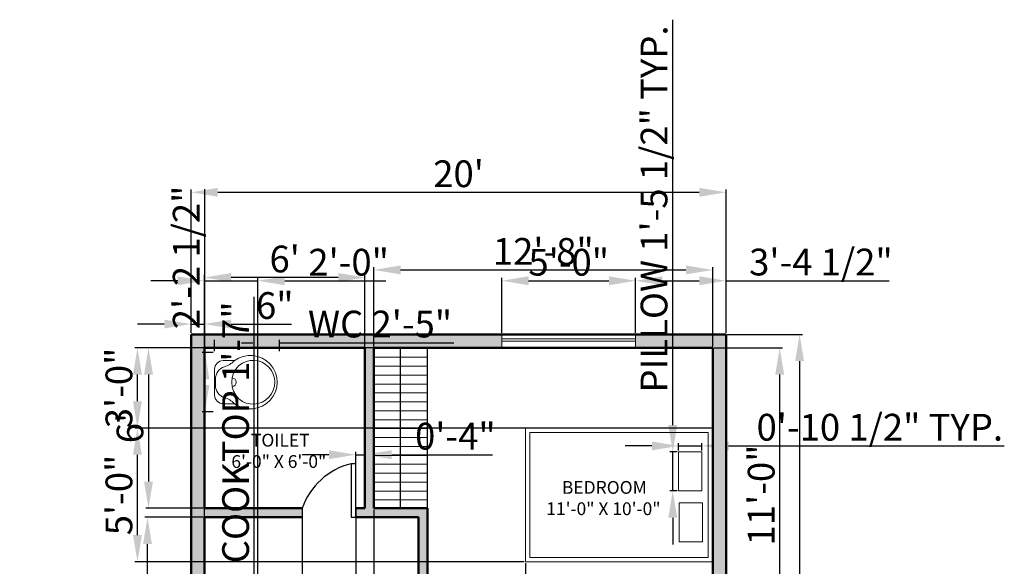
# Model space of a CAD drawing. Units: inches. Extents: x 2549 to 2991, y 1646 to 2183.
# Tile 3 of 3: x 2549 to 2991, y 1938 to 2183. Entities that reach past the tile are written whole.
import ezdxf

# ---------------------------------------------------------------- set-up
doc = ezdxf.new("R2010")
doc.units = ezdxf.units.IN
for name, color, linetype, lineweight in [('A-ANNO-DIMS', 2, 'Continuous', 18), ('A-AREA-IDEN', 7, 'Continuous', 25), ('A-DOOR', 3, 'Continuous', 25), ('A-FLOR-CASE', 8, 'Continuous', 25), ('A-FLOR-FIXT', 8, 'Continuous', 20), ('A-FLOR-PATT', 9, 'Continuous', 13), ('A-FURN', 9, 'Continuous', 18), ('A-GLAZ', 4, 'Continuous', 18), ('A-WALL', 7, 'Continuous', 50)]:
    doc.layers.add(name, color=color, linetype=linetype, lineweight=lineweight)
doc.layers.add('A-WALL-PATT', color=251, linetype='Continuous', lineweight=13, true_color=0x636466)
doc.styles.get("Standard").update_dxf_attribs({"font": 'arial.ttf'})
doc.dimstyles.new('ISO-25', dxfattribs={"dimtxt": 12, "dimasz": 12, "dimexe": 1.25, "dimexo": 0.625, "dimtad": 1, "dimlunit": 3, "dimtxsty": 'Standard', "dimcen": 2.5, "dimadec": 0, "dimazin": 0, "dimtfac": 1, "dimtmove": 0, "dimatfit": 3, "dimfxl": 1, "dimarcsym": 0})

# ---------------------------------------------------------------- blocks, each defined once
blk = doc.blocks.new('A$C6EF51710')
at = {"linetype": 'ByBlock'}
for p, q in [((0, 0.0811), (0, 0.2335)), ((0.0508, 0.2843), (0.1169, 0.2843)), ((0.0041, 0.1392), (0.0041, 0.1755)), ((0.1169, 0.0303), (0.0508, 0.0303))]:
    blk.add_line(p, q, dxfattribs=at)
for centre, radius, start, end in [((0.2107, 0.1573), 0.1576, 232.89836, 127.10164), ((0.0508, 0.2335), 0.0508, 90, 180), ((0.0803, 0.1755), 0.0762, 107.10464, 180), ((0.0168, 0.3818), 0.1397, 287.10464, 315), ((0.2413, 0.1573), 0.1397, 135, 225), ((0.2254, 0.1573), 0.1289, 230.00836, 129.99164), ((0.1016, 0.1573), 0.0254, 275.21591, 84.78409), ((0.0803, 0.1392), 0.0762, 180, 252.89536), ((0.0508, 0.0811), 0.0508, 180, 270), ((0.0168, -0.0672), 0.1397, 45, 72.89536)]:
    blk.add_arc(centre, radius, start, end, dxfattribs=at)
blk = doc.blocks.new('*D5')
at = {"layer": 'A-ANNO-DIMS', "color": 0, "lineweight": -2, "transparency": 16777216}
for p, q in [((2866.66, 2042.26), (2900.26, 2042.26)), ((2899.01, 2030.26), (2899.01, 1694.26)), ((2866.66, 1682.26), (2900.26, 1682.26))]:
    blk.add_line(p, q, dxfattribs=at)
at = {"layer": 'A-ANNO-DIMS', "color": 0, "transparency": 16777216}
for points in [[(2897.01, 2030.26), (2901.01, 2030.26), (2899.01, 2042.26)], [(2897.01, 1694.26), (2901.01, 1694.26), (2899.01, 1682.26)]]:
    blk.add_solid(points, dxfattribs=at)
at = {"layer": 'Defpoints', "color": 0, "transparency": 16777216}
for p in [(2866.04, 2042.26), (2866.04, 1682.26), (2899.01, 1682.26)]:
    blk.add_point(p, dxfattribs=at)
at = {"layer": 'A-ANNO-DIMS', "color": 0, "transparency": 16777216, "insert": (2892.25, 1862.26), "char_height": 12, "attachment_point": 5, "rotation": 90}
blk.add_mtext("30'", dxfattribs=at)
blk = doc.blocks.new('*D6')
at = {"layer": 'A-ANNO-DIMS', "color": 0, "lineweight": -2, "transparency": 16777216}
for p, q in [((2626.04, 2042.89), (2626.04, 2107.23)), ((2866.04, 2042.89), (2866.04, 2107.23)), ((2638.04, 2105.98), (2854.04, 2105.98))]:
    blk.add_line(p, q, dxfattribs=at)
at = {"layer": 'A-ANNO-DIMS', "color": 0, "transparency": 16777216}
for points in [[(2638.04, 2107.98), (2638.04, 2103.98), (2626.04, 2105.98)], [(2854.04, 2107.98), (2854.04, 2103.98), (2866.04, 2105.98)]]:
    blk.add_solid(points, dxfattribs=at)
at = {"layer": 'Defpoints', "color": 0, "transparency": 16777216}
for p in [(2866.04, 2105.98), (2626.04, 2042.26), (2866.04, 2042.26)]:
    blk.add_point(p, dxfattribs=at)
at = {"layer": 'A-ANNO-DIMS', "color": 0, "transparency": 16777216, "insert": (2746.04, 2112.74), "char_height": 12, "attachment_point": 5}
blk.add_mtext("20'", dxfattribs=at)
blk = doc.blocks.new('*D7')
at = {"layer": 'A-ANNO-DIMS', "color": 0, "lineweight": -2, "transparency": 16777216}
for p, q in [((2708.04, 2036.89), (2708.04, 2072.42)), ((2860.04, 2036.89), (2860.04, 2072.42)), ((2720.04, 2071.17), (2848.04, 2071.17))]:
    blk.add_line(p, q, dxfattribs=at)
at = {"layer": 'A-ANNO-DIMS', "color": 0, "transparency": 16777216}
for points in [[(2720.04, 2073.17), (2720.04, 2069.17), (2708.04, 2071.17)], [(2848.04, 2073.17), (2848.04, 2069.17), (2860.04, 2071.17)]]:
    blk.add_solid(points, dxfattribs=at)
at = {"layer": 'Defpoints', "color": 0, "transparency": 16777216}
for p in [(2860.04, 2071.17), (2708.04, 2036.26), (2860.04, 2036.26)]:
    blk.add_point(p, dxfattribs=at)
at = {"layer": 'A-ANNO-DIMS', "color": 0, "transparency": 16777216, "insert": (2784.04, 2077.93), "char_height": 12, "attachment_point": 5}
blk.add_mtext('12\'-8"', dxfattribs=at)
blk = doc.blocks.new('*D8')
at = {"layer": 'A-ANNO-DIMS', "color": 0, "lineweight": -2, "transparency": 16777216}
for p, q in [((2632.04, 2036.89), (2632.04, 2069.02)), ((2692.04, 2067.77), (2644.04, 2067.77)), ((2704.04, 2036.89), (2704.04, 2069.02))]:
    blk.add_line(p, q, dxfattribs=at)
at = {"layer": 'A-ANNO-DIMS', "color": 0, "transparency": 16777216}
for points in [[(2644.04, 2069.77), (2644.04, 2065.77), (2632.04, 2067.77)], [(2692.04, 2069.77), (2692.04, 2065.77), (2704.04, 2067.77)]]:
    blk.add_solid(points, dxfattribs=at)
at = {"layer": 'Defpoints', "color": 0, "transparency": 16777216}
for p in [(2632.04, 2067.77), (2632.04, 2036.26), (2704.04, 2036.26)]:
    blk.add_point(p, dxfattribs=at)
at = {"layer": 'A-ANNO-DIMS', "color": 0, "transparency": 16777216, "insert": (2668.04, 2074.52), "char_height": 12, "attachment_point": 5}
blk.add_mtext("6'", dxfattribs=at)
blk = doc.blocks.new('*D9')
at = {"layer": 'A-ANNO-DIMS', "color": 0, "lineweight": -2, "transparency": 16777216}
for p, q in [((2614.04, 2046.9), (2602.04, 2046.9)), ((2626.04, 2042.89), (2626.04, 2048.15)), ((2626.04, 2046.9), (2632.04, 2046.9)), ((2632.04, 2042.89), (2632.04, 2048.15)), ((2644.04, 2046.9), (2671.15, 2046.9))]:
    blk.add_line(p, q, dxfattribs=at)
at = {"layer": 'A-ANNO-DIMS', "color": 0, "transparency": 16777216}
for points in [[(2614.04, 2048.9), (2614.04, 2044.9), (2626.04, 2046.9)], [(2644.04, 2048.9), (2644.04, 2044.9), (2632.04, 2046.9)]]:
    blk.add_solid(points, dxfattribs=at)
at = {"layer": 'Defpoints', "color": 0, "transparency": 16777216}
for p in [(2632.04, 2046.9), (2626.04, 2042.26), (2632.04, 2042.26)]:
    blk.add_point(p, dxfattribs=at)
at = {"layer": 'A-ANNO-DIMS', "color": 0, "transparency": 16777216, "insert": (2663.59, 2053.65), "char_height": 12, "attachment_point": 5}
blk.add_mtext('6"', dxfattribs=at)
blk = doc.blocks.new('*D10')
at = {"layer": 'A-ANNO-DIMS', "color": 0, "lineweight": -2, "transparency": 16777216}
for p, q in [((2631.41, 2036.26), (2605.7, 2036.26)), ((2606.95, 2024.26), (2606.95, 1976.26)), ((2631.41, 1964.26), (2605.7, 1964.26))]:
    blk.add_line(p, q, dxfattribs=at)
at = {"layer": 'A-ANNO-DIMS', "color": 0, "transparency": 16777216}
for points in [[(2604.95, 2024.26), (2608.95, 2024.26), (2606.95, 2036.26)], [(2604.95, 1976.26), (2608.95, 1976.26), (2606.95, 1964.26)]]:
    blk.add_solid(points, dxfattribs=at)
at = {"layer": 'Defpoints', "color": 0, "transparency": 16777216}
for p in [(2632.04, 2036.26), (2606.95, 1964.26), (2632.04, 1964.26)]:
    blk.add_point(p, dxfattribs=at)
at = {"layer": 'A-ANNO-DIMS', "color": 0, "transparency": 16777216, "insert": (2600.19, 2000.26), "char_height": 12, "attachment_point": 5, "rotation": 90}
blk.add_mtext("6'", dxfattribs=at)
blk = doc.blocks.new('*D11')
at = {"layer": 'A-ANNO-DIMS', "color": 0, "lineweight": -2, "transparency": 16777216}
for p, q in [((2631.41, 1960.26), (2605.25, 1960.26)), ((2606.5, 1832.26), (2606.5, 1948.26)), ((2631.41, 1820.26), (2605.25, 1820.26))]:
    blk.add_line(p, q, dxfattribs=at)
at = {"layer": 'A-ANNO-DIMS', "color": 0, "transparency": 16777216}
for points in [[(2604.5, 1948.26), (2608.5, 1948.26), (2606.5, 1960.26)], [(2604.5, 1832.26), (2608.5, 1832.26), (2606.5, 1820.26)]]:
    blk.add_solid(points, dxfattribs=at)
at = {"layer": 'Defpoints', "color": 0, "transparency": 16777216}
for p in [(2606.5, 1960.26), (2632.04, 1960.26), (2632.04, 1820.26)]:
    blk.add_point(p, dxfattribs=at)
at = {"layer": 'A-ANNO-DIMS', "color": 0, "transparency": 16777216, "insert": (2599.75, 1890.26), "char_height": 12, "attachment_point": 5, "rotation": 90}
blk.add_mtext('11\'-8"', dxfattribs=at)
blk = doc.blocks.new('BED-PILLOW')
blk.add_lwpolyline([(0, 17.55), (10.43, 17.55), (10.43, 0), (0, 0)], close=True)
blk = doc.blocks.new('*D20')
at = {"layer": 'A-ANNO-DIMS', "color": 0, "lineweight": -2, "transparency": 16777216}
for p, q in [((2842.11, 2001.62), (2842.11, 2183.39)), ((2844.12, 1989.62), (2840.86, 1989.62)), ((2842.11, 1972.07), (2842.11, 1989.62)), ((2844.12, 1972.07), (2840.86, 1972.07)), ((2842.11, 1960.07), (2842.11, 1948.07))]:
    blk.add_line(p, q, dxfattribs=at)
at = {"layer": 'A-ANNO-DIMS', "color": 0, "transparency": 16777216}
for points in [[(2840.11, 2001.62), (2844.11, 2001.62), (2842.11, 1989.62)], [(2840.11, 1960.07), (2844.11, 1960.07), (2842.11, 1972.07)]]:
    blk.add_solid(points, dxfattribs=at)
at = {"layer": 'Defpoints', "color": 0, "transparency": 16777216}
for p in [(2842.11, 1989.62), (2844.74, 1989.62), (2844.74, 1972.07)]:
    blk.add_point(p, dxfattribs=at)
at = {"layer": 'A-ANNO-DIMS', "color": 0, "transparency": 16777216, "insert": (2835.28, 2098.5), "char_height": 12, "attachment_point": 5, "rotation": 90}
blk.add_mtext('PILLOW 1\'-5 1/2" TYP.', dxfattribs=at)
blk = doc.blocks.new('*D21')
at = {"layer": 'A-ANNO-DIMS', "color": 0, "lineweight": -2, "transparency": 16777216}
for p, q in [((2832.74, 1992.25), (2820.74, 1992.25)), ((2844.74, 1990.25), (2844.74, 1993.5)), ((2844.74, 1992.25), (2855.17, 1992.25)), ((2855.17, 1990.25), (2855.17, 1993.5)), ((2867.17, 1992.25), (2990.85, 1992.25))]:
    blk.add_line(p, q, dxfattribs=at)
at = {"layer": 'A-ANNO-DIMS', "color": 0, "transparency": 16777216}
for points in [[(2832.74, 1994.25), (2832.74, 1990.25), (2844.74, 1992.25)], [(2867.17, 1994.25), (2867.17, 1990.25), (2855.17, 1992.25)]]:
    blk.add_solid(points, dxfattribs=at)
at = {"layer": 'Defpoints', "color": 0, "transparency": 16777216}
for p in [(2855.17, 1992.25), (2844.74, 1989.62), (2855.17, 1989.62)]:
    blk.add_point(p, dxfattribs=at)
at = {"layer": 'A-ANNO-DIMS', "color": 0, "transparency": 16777216, "insert": (2935.01, 1999.08), "char_height": 12, "attachment_point": 5}
blk.add_mtext('0\'-10 1/2" TYP.', dxfattribs=at)
blk = doc.blocks.new('*D24')
at = {"layer": 'A-ANNO-DIMS', "color": 0, "lineweight": -2, "transparency": 16777216}
for p, q in [((2654.4, 1925.59), (2654.4, 2059.08)), ((2652.15, 1913.59), (2655.65, 1913.59)), ((2654.4, 1894.39), (2654.4, 1913.59)), ((2652.15, 1894.39), (2655.65, 1894.39)), ((2654.4, 1882.39), (2654.4, 1870.39))]:
    blk.add_line(p, q, dxfattribs=at)
at = {"layer": 'A-ANNO-DIMS', "color": 0, "transparency": 16777216}
for points in [[(2652.4, 1925.59), (2656.4, 1925.59), (2654.4, 1913.59)], [(2652.4, 1882.39), (2656.4, 1882.39), (2654.4, 1894.39)]]:
    blk.add_solid(points, dxfattribs=at)
at = {"layer": 'Defpoints', "color": 0, "transparency": 16777216}
for p in [(2651.52, 1913.59), (2654.4, 1913.59), (2651.52, 1894.39)]:
    blk.add_point(p, dxfattribs=at)
at = {"layer": 'A-ANNO-DIMS', "color": 0, "transparency": 16777216, "insert": (2647.57, 1998.33), "char_height": 12, "attachment_point": 5, "rotation": 90}
blk.add_mtext('COOKTOP 1\'-7"', dxfattribs=at)
blk = doc.blocks.new('*D25')
at = {"layer": 'A-ANNO-DIMS', "color": 0, "lineweight": -2, "transparency": 16777216}
for p, q in [((2633.92, 1914.21), (2633.92, 1917.72)), ((2651.52, 1914.21), (2651.52, 1917.72)), ((2621.92, 1916.47), (2549.94, 1916.47)), ((2651.52, 1916.47), (2633.92, 1916.47)), ((2663.52, 1916.47), (2675.52, 1916.47))]:
    blk.add_line(p, q, dxfattribs=at)
at = {"layer": 'A-ANNO-DIMS', "color": 0, "transparency": 16777216}
for points in [[(2621.92, 1918.47), (2621.92, 1914.47), (2633.92, 1916.47)], [(2663.52, 1918.47), (2663.52, 1914.47), (2651.52, 1916.47)]]:
    blk.add_solid(points, dxfattribs=at)
at = {"layer": 'Defpoints', "color": 0, "transparency": 16777216}
for p in [(2633.92, 1916.47), (2633.92, 1913.59), (2651.52, 1913.59)]:
    blk.add_point(p, dxfattribs=at)
at = {"layer": 'A-ANNO-DIMS', "color": 0, "transparency": 16777216, "insert": (2579.93, 1923.3), "char_height": 12, "attachment_point": 5}
blk.add_mtext('1\'-5 1/2"', dxfattribs=at)
blk = doc.blocks.new('*D26')
at = {"layer": 'A-ANNO-DIMS', "color": 0, "lineweight": -2, "transparency": 16777216}
for p, q in [((2636.61, 2034.77), (2636.61, 2039.76)), ((2648.61, 2038.51), (2653.7, 2038.51)), ((2665.7, 2034.77), (2665.7, 2039.76)), ((2665.7, 2038.51), (2743.93, 2038.51))]:
    blk.add_line(p, q, dxfattribs=at)
at = {"layer": 'A-ANNO-DIMS', "color": 0, "transparency": 16777216}
for points in [[(2648.61, 2040.51), (2648.61, 2036.51), (2636.61, 2038.51)], [(2653.7, 2040.51), (2653.7, 2036.51), (2665.7, 2038.51)]]:
    blk.add_solid(points, dxfattribs=at)
at = {"layer": 'Defpoints', "color": 0, "transparency": 16777216}
for p in [(2665.7, 2038.51), (2636.61, 2034.14), (2665.7, 2034.14)]:
    blk.add_point(p, dxfattribs=at)
at = {"layer": 'A-ANNO-DIMS', "color": 0, "transparency": 16777216, "insert": (2710.82, 2045.34), "char_height": 12, "attachment_point": 5}
blk.add_mtext('WC 2\'-5"', dxfattribs=at)
blk = doc.blocks.new('*D27')
at = {"layer": 'A-ANNO-DIMS', "color": 0, "lineweight": -2, "transparency": 16777216}
for p, q in [((2632.25, 2034.14), (2632.25, 2107.46)), ((2635.99, 2034.14), (2631, 2034.14)), ((2632.25, 2019.52), (2632.25, 2022.14)), ((2635.99, 2007.52), (2631, 2007.52))]:
    blk.add_line(p, q, dxfattribs=at)
at = {"layer": 'A-ANNO-DIMS', "color": 0, "transparency": 16777216}
for points in [[(2630.25, 2022.14), (2634.25, 2022.14), (2632.25, 2034.14)], [(2630.25, 2019.52), (2634.25, 2019.52), (2632.25, 2007.52)]]:
    blk.add_solid(points, dxfattribs=at)
at = {"layer": 'Defpoints', "color": 0, "transparency": 16777216}
for p in [(2632.25, 2034.14), (2636.61, 2034.14), (2636.61, 2007.52)]:
    blk.add_point(p, dxfattribs=at)
at = {"layer": 'A-ANNO-DIMS', "color": 0, "transparency": 16777216, "insert": (2625.42, 2076.8), "char_height": 12, "attachment_point": 5, "rotation": 90}
blk.add_mtext('2\'-2 1/2"', dxfattribs=at)
blk = doc.blocks.new('*D31')
at = {"layer": 'A-ANNO-DIMS', "color": 0, "lineweight": -2, "transparency": 16777216}
for p, q in [((2765.46, 2042.89), (2765.46, 2067.56)), ((2825.46, 2042.89), (2825.46, 2067.56)), ((2777.46, 2066.31), (2813.46, 2066.31))]:
    blk.add_line(p, q, dxfattribs=at)
at = {"layer": 'A-ANNO-DIMS', "color": 0, "transparency": 16777216}
for points in [[(2777.46, 2068.31), (2777.46, 2064.31), (2765.46, 2066.31)], [(2813.46, 2068.31), (2813.46, 2064.31), (2825.46, 2066.31)]]:
    blk.add_solid(points, dxfattribs=at)
at = {"layer": 'Defpoints', "color": 0, "transparency": 16777216}
for p in [(2825.46, 2066.31), (2765.46, 2042.26), (2825.46, 2042.26)]:
    blk.add_point(p, dxfattribs=at)
at = {"layer": 'A-ANNO-DIMS', "color": 0, "transparency": 16777216, "insert": (2795.46, 2073.07), "char_height": 12, "attachment_point": 5}
blk.add_mtext('5\'-0"', dxfattribs=at)
blk = doc.blocks.new('*D32')
at = {"layer": 'A-ANNO-DIMS', "color": 0, "lineweight": -2, "transparency": 16777216}
for p, q in [((2825.46, 2042.89), (2825.46, 2067.56)), ((2866.04, 2042.89), (2866.04, 2067.56)), ((2837.46, 2066.31), (2854.04, 2066.31)), ((2866.04, 2066.31), (2939.14, 2066.31))]:
    blk.add_line(p, q, dxfattribs=at)
at = {"layer": 'A-ANNO-DIMS', "color": 0, "transparency": 16777216}
for points in [[(2837.46, 2068.31), (2837.46, 2064.31), (2825.46, 2066.31)], [(2854.04, 2068.31), (2854.04, 2064.31), (2866.04, 2066.31)]]:
    blk.add_solid(points, dxfattribs=at)
at = {"layer": 'Defpoints', "color": 0, "transparency": 16777216}
for p in [(2866.04, 2066.31), (2825.46, 2042.26), (2866.04, 2042.26)]:
    blk.add_point(p, dxfattribs=at)
at = {"layer": 'A-ANNO-DIMS', "color": 0, "transparency": 16777216, "insert": (2908.59, 2073.15), "char_height": 12, "attachment_point": 5}
blk.add_mtext('3\'-4 1/2"', dxfattribs=at)
blk = doc.blocks.new('*D33')
at = {"layer": 'A-ANNO-DIMS', "color": 0, "lineweight": -2, "transparency": 16777216}
for p, q in [((2675.89, 1963.64), (2675.89, 1656.96)), ((2699.89, 1963.64), (2699.89, 1656.96)), ((2663.89, 1658.21), (2651.89, 1658.21)), ((2675.89, 1658.21), (2699.89, 1658.21)), ((2711.89, 1658.21), (2757.24, 1658.21))]:
    blk.add_line(p, q, dxfattribs=at)
at = {"layer": 'A-ANNO-DIMS', "color": 0, "transparency": 16777216}
for points in [[(2663.89, 1660.21), (2663.89, 1656.21), (2675.89, 1658.21)], [(2711.89, 1660.21), (2711.89, 1656.21), (2699.89, 1658.21)]]:
    blk.add_solid(points, dxfattribs=at)
at = {"layer": 'Defpoints', "color": 0, "transparency": 16777216}
for p in [(2675.89, 1964.26), (2699.89, 1964.26), (2699.89, 1658.21)]:
    blk.add_point(p, dxfattribs=at)
at = {"layer": 'A-ANNO-DIMS', "color": 0, "transparency": 16777216, "insert": (2740.57, 1664.97), "char_height": 12, "attachment_point": 5}
blk.add_mtext('2\'-0"', dxfattribs=at)
blk = doc.blocks.new('*D34')
at = {"layer": 'A-ANNO-DIMS', "color": 0, "lineweight": -2, "transparency": 16777216}
for p, q in [((2687.89, 1988.31), (2675.89, 1988.31)), ((2699.89, 1964.89), (2699.89, 1989.56)), ((2699.89, 1988.31), (2704.04, 1988.31)), ((2704.04, 1964.89), (2704.04, 1989.56)), ((2716.04, 1988.31), (2761.19, 1988.31))]:
    blk.add_line(p, q, dxfattribs=at)
at = {"layer": 'A-ANNO-DIMS', "color": 0, "transparency": 16777216}
for points in [[(2687.89, 1990.31), (2687.89, 1986.31), (2699.89, 1988.31)], [(2716.04, 1990.31), (2716.04, 1986.31), (2704.04, 1988.31)]]:
    blk.add_solid(points, dxfattribs=at)
at = {"layer": 'Defpoints', "color": 0, "transparency": 16777216}
for p in [(2704.04, 1988.31), (2699.89, 1964.26), (2704.04, 1964.26)]:
    blk.add_point(p, dxfattribs=at)
at = {"layer": 'A-ANNO-DIMS', "color": 0, "transparency": 16777216, "insert": (2744.61, 1995.07), "char_height": 12, "attachment_point": 5}
blk.add_mtext('0\'-4"', dxfattribs=at)
blk = doc.blocks.new('*D41')
at = {"layer": 'A-ANNO-DIMS', "color": 0, "lineweight": -2, "transparency": 16777216}
for p, q in [((2632.04, 1820.89), (2632.04, 2067.56)), ((2656.04, 1820.89), (2656.04, 2067.56)), ((2620.04, 2066.31), (2608.04, 2066.31)), ((2632.04, 2066.31), (2656.04, 2066.31)), ((2668.04, 2066.31), (2713.39, 2066.31))]:
    blk.add_line(p, q, dxfattribs=at)
at = {"layer": 'A-ANNO-DIMS', "color": 0, "transparency": 16777216}
for points in [[(2620.04, 2068.31), (2620.04, 2064.31), (2632.04, 2066.31)], [(2668.04, 2068.31), (2668.04, 2064.31), (2656.04, 2066.31)]]:
    blk.add_solid(points, dxfattribs=at)
at = {"layer": 'Defpoints', "color": 0, "transparency": 16777216}
for p in [(2656.04, 2066.31), (2632.04, 1820.26), (2656.04, 1820.26)]:
    blk.add_point(p, dxfattribs=at)
at = {"layer": 'A-ANNO-DIMS', "color": 0, "transparency": 16777216, "insert": (2696.72, 2073.07), "char_height": 12, "attachment_point": 5}
blk.add_mtext('2\'-0"', dxfattribs=at)
blk = doc.blocks.new('*D42')
at = {"layer": 'A-ANNO-DIMS', "color": 0, "lineweight": -2, "transparency": 16777216}
for p, q in [((2776.04, 1939.64), (2776.04, 1656.96)), ((2860.04, 1939.64), (2860.04, 1656.96)), ((2788.04, 1658.21), (2848.04, 1658.21))]:
    blk.add_line(p, q, dxfattribs=at)
at = {"layer": 'A-ANNO-DIMS', "color": 0, "transparency": 16777216}
for points in [[(2788.04, 1660.21), (2788.04, 1656.21), (2776.04, 1658.21)], [(2848.04, 1660.21), (2848.04, 1656.21), (2860.04, 1658.21)]]:
    blk.add_solid(points, dxfattribs=at)
at = {"layer": 'Defpoints', "color": 0, "transparency": 16777216}
for p in [(2776.04, 1940.26), (2860.04, 1940.26), (2860.04, 1658.21)]:
    blk.add_point(p, dxfattribs=at)
at = {"layer": 'A-ANNO-DIMS', "color": 0, "transparency": 16777216, "insert": (2818.04, 1664.97), "char_height": 12, "attachment_point": 5}
blk.add_mtext('7\'-0"', dxfattribs=at)
blk = doc.blocks.new('*D43')
at = {"layer": 'A-ANNO-DIMS', "color": 0, "lineweight": -2, "transparency": 16777216}
for p, q in [((2775.41, 2000.26), (2600.74, 2000.26)), ((2601.99, 1952.26), (2601.99, 1988.26)), ((2775.41, 1940.26), (2600.74, 1940.26))]:
    blk.add_line(p, q, dxfattribs=at)
at = {"layer": 'A-ANNO-DIMS', "color": 0, "transparency": 16777216}
for points in [[(2599.99, 1988.26), (2603.99, 1988.26), (2601.99, 2000.26)], [(2599.99, 1952.26), (2603.99, 1952.26), (2601.99, 1940.26)]]:
    blk.add_solid(points, dxfattribs=at)
at = {"layer": 'Defpoints', "color": 0, "transparency": 16777216}
for p in [(2601.99, 2000.26), (2776.04, 2000.26), (2776.04, 1940.26)]:
    blk.add_point(p, dxfattribs=at)
at = {"layer": 'A-ANNO-DIMS', "color": 0, "transparency": 16777216, "insert": (2595.24, 1970.26), "char_height": 12, "attachment_point": 5, "rotation": 90}
blk.add_mtext('5\'-0"', dxfattribs=at)
blk = doc.blocks.new('*D44')
at = {"layer": 'A-ANNO-DIMS', "color": 0, "lineweight": -2, "transparency": 16777216}
for p, q in [((2708.04, 1963.64), (2708.04, 1656.96)), ((2732.04, 1963.64), (2732.04, 1656.96)), ((2696.04, 1658.21), (2684.04, 1658.21)), ((2708.04, 1658.21), (2732.04, 1658.21)), ((2744.04, 1658.21), (2789.39, 1658.21))]:
    blk.add_line(p, q, dxfattribs=at)
at = {"layer": 'A-ANNO-DIMS', "color": 0, "transparency": 16777216}
for points in [[(2696.04, 1660.21), (2696.04, 1656.21), (2708.04, 1658.21)], [(2744.04, 1660.21), (2744.04, 1656.21), (2732.04, 1658.21)]]:
    blk.add_solid(points, dxfattribs=at)
at = {"layer": 'Defpoints', "color": 0, "transparency": 16777216}
for p in [(2708.04, 1964.26), (2732.04, 1964.26), (2732.04, 1658.21)]:
    blk.add_point(p, dxfattribs=at)
at = {"layer": 'A-ANNO-DIMS', "color": 0, "transparency": 16777216, "insert": (2772.72, 1664.97), "char_height": 12, "attachment_point": 5}
blk.add_mtext('2\'-0"', dxfattribs=at)
blk = doc.blocks.new('*D45')
at = {"layer": 'A-ANNO-DIMS', "color": 0, "lineweight": -2, "transparency": 16777216}
for p, q in [((2860.66, 2036.26), (2891.34, 2036.26)), ((2890.09, 1916.26), (2890.09, 2024.26)), ((2860.66, 1904.26), (2891.34, 1904.26))]:
    blk.add_line(p, q, dxfattribs=at)
at = {"layer": 'A-ANNO-DIMS', "color": 0, "transparency": 16777216}
for points in [[(2888.09, 2024.26), (2892.09, 2024.26), (2890.09, 2036.26)], [(2888.09, 1916.26), (2892.09, 1916.26), (2890.09, 1904.26)]]:
    blk.add_solid(points, dxfattribs=at)
at = {"layer": 'Defpoints', "color": 0, "transparency": 16777216}
for p in [(2860.04, 2036.26), (2890.09, 2036.26), (2860.04, 1904.26)]:
    blk.add_point(p, dxfattribs=at)
at = {"layer": 'A-ANNO-DIMS', "color": 0, "transparency": 16777216, "insert": (2883.34, 1970.26), "char_height": 12, "attachment_point": 5, "rotation": 90}
blk.add_mtext('11\'-0"', dxfattribs=at)
blk = doc.blocks.new('*D46')
at = {"layer": 'A-ANNO-DIMS', "color": 0, "lineweight": -2, "transparency": 16777216}
for p, q in [((2859.41, 2036.26), (2600.74, 2036.26)), ((2601.99, 2012.26), (2601.99, 2024.26)), ((2859.41, 2000.26), (2600.74, 2000.26))]:
    blk.add_line(p, q, dxfattribs=at)
at = {"layer": 'A-ANNO-DIMS', "color": 0, "transparency": 16777216}
for points in [[(2599.99, 2024.26), (2603.99, 2024.26), (2601.99, 2036.26)], [(2599.99, 2012.26), (2603.99, 2012.26), (2601.99, 2000.26)]]:
    blk.add_solid(points, dxfattribs=at)
at = {"layer": 'Defpoints', "color": 0, "transparency": 16777216}
for p in [(2601.99, 2036.26), (2860.04, 2036.26), (2860.04, 2000.26)]:
    blk.add_point(p, dxfattribs=at)
at = {"layer": 'A-ANNO-DIMS', "color": 0, "transparency": 16777216, "insert": (2595.23, 2018.26), "char_height": 12, "attachment_point": 5, "rotation": 90}
blk.add_mtext('3\'-0"', dxfattribs=at)

msp = doc.modelspace()

# ---------------------------------------------------------------- hatches: boundary and pattern name
at = {"layer": 'A-FLOR-PATT'}
h = msp.add_hatch(dxfattribs=at)
h.set_pattern_fill('ANSI31', color=256, scale=1.259843, angle=-45, style=0)
h.paths.add_polyline_path([(2708.038, 1964.264), (2732.038, 1964.264), (2732.038, 2036.264), (2708.038, 2036.264)])
at = {"layer": 'A-WALL-PATT'}
h = msp.add_hatch(color=256, dxfattribs=at)
h.dxf.hatch_style = 1
h.paths.add_polyline_path([(2765.46, 2042.264), (2626.038, 2042.264), (2626.038, 1682.264), (2673.991, 1682.264), (2673.991, 1688.264), (2632.038, 1688.264), (2632.038, 1816.264), (2752.038, 1816.264), (2752.038, 1811.649), (2756.038, 1811.649), (2756.038, 1820.264), (2632.038, 1820.264), (2632.038, 1960.264), (2675.89, 1960.264), (2675.89, 1964.264), (2632.038, 1964.264), (2632.038, 2036.264), (2704.038, 2036.264), (2704.038, 1964.264), (2699.89, 1964.264), (2699.89, 1960.264), (2728.038, 1960.264), (2728.038, 1900.264), (2734.981, 1900.264), (2734.981, 1904.264), (2732.038, 1904.264), (2732.038, 1964.264), (2708.038, 1964.264), (2708.038, 2036.264), (2765.46, 2036.264)])
h.paths.add_polyline_path([(2866.038, 2042.264), (2825.46, 2042.264), (2825.46, 2036.264), (2860.038, 2036.264), (2860.038, 1904.264), (2770.981, 1904.264), (2770.981, 1900.264), (2860.038, 1900.264), (2860.038, 1688.264), (2852.256, 1688.264), (2852.256, 1682.264), (2866.038, 1682.264)])
h.paths.add_polyline_path([(2816.256, 1688.264), (2756.038, 1688.264), (2756.038, 1775.649), (2752.038, 1775.649), (2752.038, 1688.264), (2721.991, 1688.264), (2721.991, 1682.264), (2816.256, 1682.264)])

# ---------------------------------------------------------------- linework, layer by layer
at = {"layer": 'A-DOOR'}
for p, q in [((2699.89, 1984.264), (2697.89, 1984.264)), ((2697.89, 1984.264), (2697.89, 1960.264)), ((2699.89, 1960.264), (2699.89, 1984.264)), ((2675.89, 1964.264), (2675.89, 1960.264)), ((2699.89, 1964.264), (2699.89, 1960.264)), ((2697.89, 1960.264), (2699.89, 1960.264))]:
    msp.add_line(p, q, dxfattribs=at)
msp.add_arc((2705.184, 1954.14), 30.994, 103.6117, 160.93568, dxfattribs=at)
at = {"layer": 'A-FLOR-CASE'}
for p, q in [((2720.038, 1964.264), (2720.038, 2036.264)), ((2732.038, 1964.264), (2732.038, 2036.264)), ((2656.038, 1820.264), (2656.038, 1960.264))]:
    msp.add_line(p, q, dxfattribs=at)
at = {"layer": 'A-FURN'}
for p, q in [((2776.038, 2000.264), (2776.038, 1940.264)), ((2776.038, 2000.264), (2860.038, 2000.264)), ((2778.038, 1998.264), (2858.038, 1998.264)), ((2778.038, 1998.264), (2778.038, 1942.264)), ((2858.038, 1998.264), (2858.038, 1942.264)), ((2776.038, 1940.264), (2860.038, 1940.264)), ((2778.038, 1942.264), (2858.038, 1942.264))]:
    msp.add_line(p, q, dxfattribs=at)
at = {"layer": 'A-GLAZ'}
for p, q in [((2765.46, 2042.264), (2765.46, 2036.264)), ((2825.46, 2042.264), (2825.46, 2036.264)), ((2765.46, 2040.264), (2825.46, 2040.264)), ((2765.46, 2039.264), (2825.46, 2039.264))]:
    msp.add_line(p, q, dxfattribs=at)
at = {"layer": 'A-WALL'}
for p, q in [((2626.038, 2042.264), (2866.038, 2042.264)), ((2626.038, 1682.264), (2626.038, 2042.264)), ((2866.038, 2042.264), (2866.038, 1682.264)), ((2632.038, 2036.264), (2704.038, 2036.264)), ((2632.038, 1964.264), (2632.038, 2036.264)), ((2704.038, 1964.264), (2704.038, 2036.264)), ((2708.038, 1964.264), (2708.038, 2036.264)), ((2708.038, 2036.264), (2860.038, 2036.264)), ((2860.038, 2036.264), (2860.038, 1904.264)), ((2632.038, 1964.264), (2675.89, 1964.264)), ((2699.89, 1964.264), (2704.038, 1964.264)), ((2708.038, 1964.264), (2732.038, 1964.264)), ((2732.038, 1964.264), (2732.038, 1904.264)), ((2632.038, 1960.264), (2675.89, 1960.264)), ((2632.038, 1820.264), (2632.038, 1960.264)), ((2699.89, 1960.264), (2728.038, 1960.264)), ((2728.038, 1960.264), (2728.038, 1900.264))]:
    msp.add_line(p, q, dxfattribs=at)

# ---------------------------------------------------------------- block references
at = {"layer": 'A-FLOR-FIXT', "xscale": 76.142993395288, "yscale": 76.142993395288, "zscale": 76.142993395288}
msp.add_blockref('A$C6EF51710', (2636.615, 2008.85), dxfattribs=at)
at = {"layer": 'A-FURN'}
for p in [(2844.743, 1972.069), (2844.998, 1949.246)]:
    msp.add_blockref('BED-PILLOW', p, dxfattribs=at)

# ---------------------------------------------------------------- texts
at = {"layer": 'A-AREA-IDEN', "char_height": 5.7375, "attachment_point": 1}
for s, insert in [('     TOILET\\P6\'-0" X 6\'-0"', (2644.125, 1997.681)), ('    BEDROOM\\P11\'-0" X 10\'-0"', (2785.381, 1976.51))]:
    msp.add_mtext_dynamic_manual_height_columns(s, width=199.71745, gutter_width=28.687, heights=[0], dxfattribs=dict(at, insert=insert))

# ---------------------------------------------------------------- dimensions: what is measured, and where the dimension line sits
at = {"layer": 'A-ANNO-DIMS'}
for base, p1, p2, text, picture, middle in [((2842.11, 1989.621), (2844.743, 1972.069), (2844.743, 1989.621), 'PILLOW <> TYP.', '*D20', (2835.277, 2098.504)), ((2654.403, 1913.587), (2651.523, 1894.387), (2651.523, 1913.587), 'COOKTOP <>', '*D24', (2647.569, 1998.335))]:
    dim = msp.add_linear_dim(base=base, p1=p1, p2=p2, angle=90, text=text, dimstyle='ISO-25', override={"dimdec": 1, "dimlfac": 1, "dimrnd": 0, "dimzin": 1, "dimdsep": 46, "dimlunit": 4, "dimfrac": 2}, dxfattribs=at)
    dim.commit()
    dim.dimension.update_dxf_attribs({"geometry": picture, "text_midpoint": middle})
for base, p1, p2, override, picture, middle in [((2866.038, 2105.983), (2626.038, 2042.264), (2866.038, 2042.264), {"dimclrd": 0, "dimclre": 0, "dimclrt": 0}, '*D6', (2746.038, 2112.735)), ((2866.038, 2066.314), (2825.46, 2042.264), (2866.038, 2042.264), {"dimdec": 1, "dimlfac": 1, "dimrnd": 0, "dimzin": 1, "dimdsep": 46, "dimlunit": 4, "dimfrac": 2}, '*D32', (2908.59, 2073.148)), ((2860.038, 2071.174), (2708.038, 2036.264), (2860.038, 2036.264), {"dimclrd": 0, "dimclre": 0, "dimclrt": 0}, '*D7', (2784.038, 2077.925)), ((2656.038, 2066.314), (2632.038, 1820.264), (2656.038, 1820.264), {"dimdec": 1, "dimlfac": 1, "dimrnd": 0, "dimzin": 1, "dimdsep": 46, "dimlunit": 4, "dimfrac": 2}, '*D41', (2696.715, 2073.066)), ((2632.038, 2067.767), (2704.038, 2036.264), (2632.038, 2036.264), {"dimclrd": 0, "dimclre": 0, "dimclrt": 0}, '*D8', (2668.038, 2074.519)), ((2825.46, 2066.314), (2765.46, 2042.264), (2825.46, 2042.264), {"dimdec": 1, "dimlfac": 1, "dimrnd": 0, "dimzin": 1, "dimdsep": 46, "dimlunit": 4, "dimfrac": 2}, '*D31', (2795.46, 2073.066)), ((2632.038, 2046.903), (2626.038, 2042.264), (2632.038, 2042.264), {"dimclrd": 0, "dimclre": 0, "dimclrt": 0}, '*D9', (2663.592, 2053.655)), ((2704.038, 1988.314), (2699.89, 1964.264), (2704.038, 1964.264), {"dimdec": 1, "dimlfac": 1, "dimrnd": 0, "dimzin": 1, "dimdsep": 46, "dimlunit": 4, "dimfrac": 2}, '*D34', (2744.613, 1995.066)), ((2699.89, 1658.214), (2675.89, 1964.264), (2699.89, 1964.264), {"dimdec": 1, "dimlfac": 1, "dimrnd": 0, "dimzin": 1, "dimdsep": 46, "dimlunit": 4, "dimfrac": 2}, '*D33', (2740.567, 1664.966)), ((2732.038, 1658.214), (2708.038, 1964.264), (2732.038, 1964.264), {"dimdec": 1, "dimlfac": 1, "dimrnd": 0, "dimzin": 1, "dimdsep": 46, "dimlunit": 4, "dimfrac": 2}, '*D44', (2772.715, 1664.966)), ((2860.038, 1658.214), (2776.038, 1940.264), (2860.038, 1940.264), {"dimdec": 1, "dimlfac": 1, "dimrnd": 0, "dimzin": 1, "dimdsep": 46, "dimlunit": 4, "dimfrac": 2}, '*D42', (2818.038, 1664.966))]:
    dim = msp.add_linear_dim(base=base, p1=p1, p2=p2, dimstyle='ISO-25', override=override, dxfattribs=at)
    dim.commit()
    dim.dimension.update_dxf_attribs({"geometry": picture, "text_midpoint": middle})
for base, p1, p2, angle, override, picture, middle in [((2632.252, 2034.144), (2636.615, 2007.515), (2636.615, 2034.144), 90, {"dimdec": 1, "dimlfac": 1, "dimrnd": 0, "dimzin": 1, "dimdsep": 46, "dimlunit": 4, "dimfrac": 2}, '*D27', (2625.422, 2076.802)), ((2899.007, 1682.264), (2866.038, 2042.264), (2866.038, 1682.264), 90, {"dimclrd": 0, "dimclre": 0, "dimclrt": 0}, '*D5', (2892.251, 1862.264)), ((2601.988, 2036.264), (2860.038, 2000.264), (2860.038, 2036.264), 90, {"dimdec": 1, "dimlfac": 1, "dimrnd": 0, "dimzin": 1, "dimdsep": 46, "dimlunit": 4, "dimfrac": 2}, '*D46', (2595.232, 2018.264)), ((2606.945, 1964.264), (2632.038, 2036.264), (2632.038, 1964.264), 90, {"dimclrd": 0, "dimclre": 0, "dimclrt": 0}, '*D10', (2600.193, 2000.264)), ((2890.088, 2036.264), (2860.038, 1904.264), (2860.038, 2036.264), 90, {"dimdec": 1, "dimlfac": 1, "dimrnd": 0, "dimzin": 1, "dimdsep": 46, "dimlunit": 4, "dimfrac": 2}, '*D45', (2883.336, 1970.264)), ((2601.988, 2000.264), (2776.038, 1940.264), (2776.038, 2000.264), 90, {"dimdec": 1, "dimlfac": 1, "dimrnd": 0, "dimzin": 1, "dimdsep": 46, "dimlunit": 4, "dimfrac": 2}, '*D43', (2595.236, 1970.264)), ((2606.503, 1960.264), (2632.038, 1820.264), (2632.038, 1960.264), 90, {"dimclrd": 0, "dimclre": 0, "dimclrt": 0}, '*D11', (2599.751, 1890.264)), ((2633.923, 1916.467), (2651.523, 1913.587), (2633.923, 1913.587), 180, {"dimdec": 1, "dimlfac": 1, "dimrnd": 0, "dimzin": 1, "dimdsep": 46, "dimlunit": 4, "dimfrac": 2}, '*D25', (2579.932, 1923.297))]:
    dim = msp.add_linear_dim(base=base, p1=p1, p2=p2, angle=angle, dimstyle='ISO-25', override=override, dxfattribs=at)
    dim.commit()
    dim.dimension.update_dxf_attribs({"geometry": picture, "text_midpoint": middle})
for base, p1, p2, text, picture, middle in [((2665.703, 2038.507), (2636.615, 2034.144), (2665.703, 2034.144), 'WC <>', '*D26', (2710.817, 2045.337)), ((2855.169, 1992.254), (2844.743, 1989.621), (2855.169, 1989.621), '<> TYP.', '*D21', (2935.01, 1999.084))]:
    dim = msp.add_linear_dim(base=base, p1=p1, p2=p2, text=text, dimstyle='ISO-25', override={"dimdec": 1, "dimlfac": 1, "dimrnd": 0, "dimzin": 1, "dimdsep": 46, "dimlunit": 4, "dimfrac": 2}, dxfattribs=at)
    dim.commit()
    dim.dimension.update_dxf_attribs({"geometry": picture, "text_midpoint": middle})

doc.saveas('drawing.dxf')
